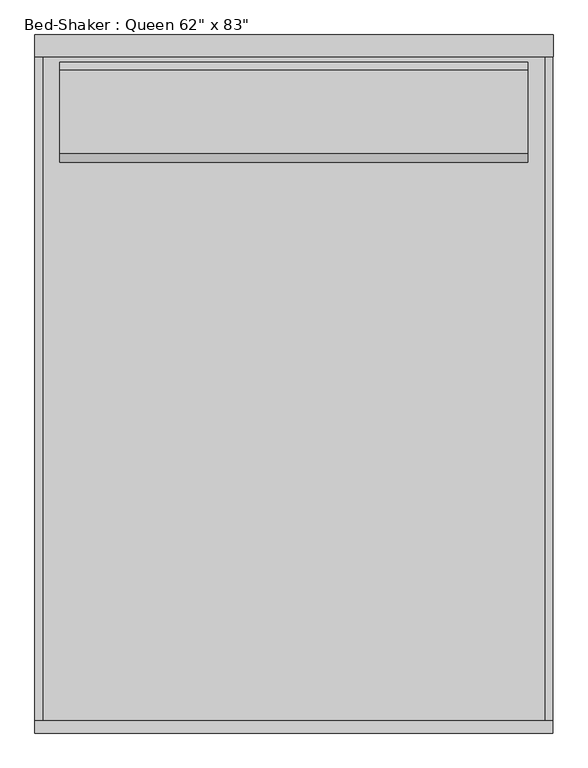
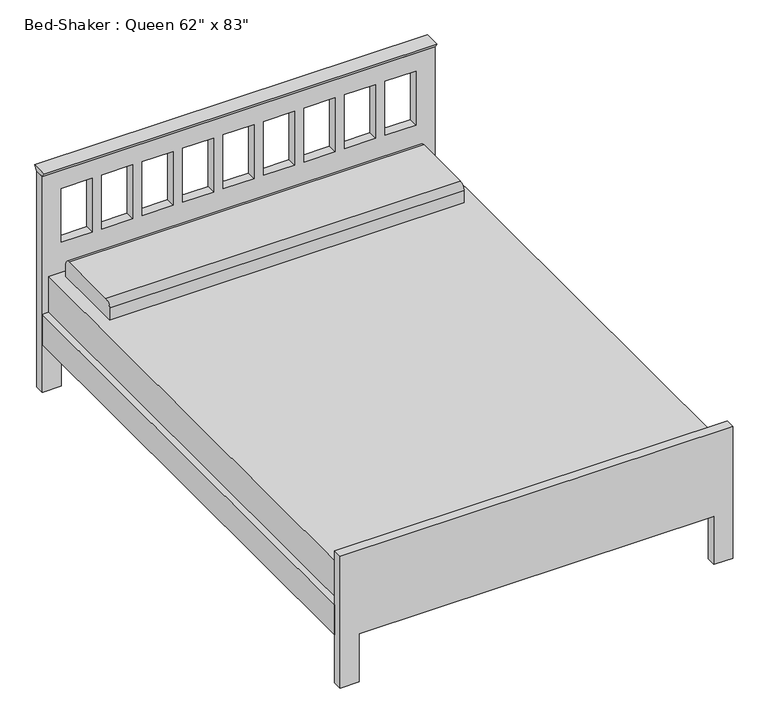
"""IFC4 building model written with IfcOpenShell, lengths in millimetres: furniture geometry."""

from ifc_helpers import new_model, si_unit, point, frame, frame_2d, origin, place, context, project, spatial, polyline, circle_curve, trimmed, segment, composite_curve, outline, extrude, source, transform, mapped, element, save


def furniture_35c09872(model_context):
    return source(origin(), model_context, "Body", "SweptSolid", [
        extrude(outline(polyline([(-38.1, 914.4), (-51.9545455, 933.45), (13.8545455, 933.45), (0.0, 914.4), (-38.1, 914.4)])), frame((-806.2365546, 0.0, 0.0), z_axis=(1.0, 0.0, 0.0), x_axis=(0.0, 1.0, 0.0)), (0.0, 0.0, 1.0), 1574.8533613),
        extrude(outline(composite_curve([segment(polyline([(-373.2486637, 482.6), (-373.2486637, 533.4)]), True, "CONTINUOUS"), segment(trimmed(circle_curve(frame_2d((-347.8486637, 533.4)), 25.4), [point((-373.2486637, 533.4))], [point((-347.8486637, 558.8))], False, "CARTESIAN"), True, "CONTINUOUS"), segment(polyline([(-347.8486637, 558.8), (-93.8486637, 558.8)]), True, "CONTINUOUS"), segment(trimmed(circle_curve(frame_2d((-93.8486637, 533.4)), 25.4), [point((-93.8486637, 558.8))], [point((-68.4486637, 533.4))], False, "CARTESIAN"), True, "CONTINUOUS"), segment(polyline([(-68.4486637, 533.4), (-68.4486637, 482.6), (-373.2486637, 482.6)]), True, "CONTINUOUS")], self_intersect=False)), frame((-730.25, 0.0, 0.0), z_axis=(1.0, 0.0, 0.0), x_axis=(0.0, 1.0, 0.0)), (0.0, 0.0, 1.0), 1422.4),
        extrude(outline(polyline([(742.95, -38.1), (742.95, -2070.1), (-781.05, -2070.1), (-781.05, -38.1), (742.95, -38.1)])), frame((0.0, 0.0, 228.6), z_axis=(0.0, 0.0, 1.0), x_axis=(1.0, 0.0, 0.0)), (0.0, 0.0, 1.0), 254.0),
        extrude(outline(polyline([(742.95, -2070.1), (742.95, -38.1), (768.35, -38.1), (768.35, -2070.1), (742.95, -2070.1)])), frame((0.0, 0.0, 203.0994861), z_axis=(0.0, 0.0, 1.0), x_axis=(1.0, 0.0, 0.0)), (0.0, 0.0, 1.0), 127.0),
        extrude(outline(polyline([(-806.45, -2070.1), (-806.45, -38.1), (-781.05, -38.1), (-781.05, -2070.1), (-806.45, -2070.1)])), frame((0.0, 0.0, 203.5755296), z_axis=(0.0, 0.0, 1.0), x_axis=(1.0, 0.0, 0.0)), (0.0, 0.0, 1.0), 127.0),
        extrude(outline(polyline([(0.0, -730.25), (203.2, -730.25), (203.2, 692.15), (0.0, 692.15), (0.0, 768.35), (558.8, 768.35), (558.8, -806.45), (0.0, -806.45), (0.0, -730.25)])), frame((0.0, -2108.2, 0.0), z_axis=(0.0, 1.0, 0.0), x_axis=(0.0, 0.0, 1.0)), (0.0, 0.0, 1.0), 38.1),
        extrude(outline(polyline([(914.4, 768.6168067), (914.4, -806.2365546), (0.0, -806.2365546), (0.0, -730.25), (203.2, -730.25), (203.2, 692.15), (0.0, 692.15), (0.0, 768.6168067), (914.4, 768.6168067)]), holes=[polyline([(838.2, -606.0722222), (609.6, -606.0722222), (609.6, -730.25), (838.2, -730.25), (838.2, -606.0722222)]), polyline([(838.2, -443.7944444), (609.6, -443.7944444), (609.6, -567.9722222), (838.2, -567.9722222), (838.2, -443.7944444)]), polyline([(838.2, -281.5166667), (609.6, -281.5166667), (609.6, -405.6944444), (838.2, -405.6944444), (838.2, -281.5166667)]), polyline([(838.2, -119.2388889), (609.6, -119.2388889), (609.6, -243.4166667), (838.2, -243.4166667), (838.2, -119.2388889)]), polyline([(838.2, 205.3166667), (609.6, 205.3166667), (609.6, 81.1388889), (838.2, 81.1388889), (838.2, 205.3166667)]), polyline([(838.2, 367.5944444), (609.6, 367.5944444), (609.6, 243.4166667), (838.2, 243.4166667), (838.2, 367.5944444)]), polyline([(838.2, 529.8722222), (609.6, 529.8722222), (609.6, 405.6944444), (838.2, 405.6944444), (838.2, 529.8722222)]), polyline([(838.2, 692.15), (609.6, 692.15), (609.6, 567.9722222), (838.2, 567.9722222), (838.2, 692.15)]), polyline([(838.2, 43.0388889), (609.6, 43.0388889), (609.6, -81.1388889), (838.2, -81.1388889), (838.2, 43.0388889)])]), frame((0.0, -38.1, 0.0), z_axis=(0.0, 1.0, 0.0), x_axis=(0.0, 0.0, 1.0)), (0.0, 0.0, 1.0), 38.1),
    ])


if __name__ == "__main__":
    model = new_model("IFC4")
    model_context = context("Model", 3, world=origin())
    ifc_project = project(units=[si_unit("LENGTHUNIT", "METRE", prefix="MILLI")], contexts=[model_context])
    site = spatial("IfcSite", under=ifc_project)
    building = spatial("IfcBuilding", under=site)
    placement = place(None, origin())
    furniture_shape = furniture_35c09872(model_context)
    element("IfcFurniture", 1, ObjectType="Bed-Shaker : Queen 62\" x 83\"", at=placement, inside=building, context=model_context, shape_type="MappedRepresentation", body=[
        mapped(furniture_shape, transform((0.0, 0.0, 0.0), x_axis=(1.0, 0.0, 0.0), y_axis=(0.0, 1.0, 0.0), z_axis=(0.0, 0.0, 1.0))),
    ])
    save(model, "model.ifc")

# Revit data of these elements
# Type "Bed-Shaker : Queen 62\" x 83\""
#   Assembly Code = "E2020200"
#   Length = 6' - 11"
#   Width = 5' - 2"
#   Frame Material = Birch
#   Mattress Material = Plywood, Sheathing
#   Default Elevation = 0
# Element 1 (IfcFurniture, "Bed-Shaker : Queen 62\" x 83\"")
#   Materials on its faces: "Birch", "Plywood, Sheathing"
# Materials
#   "Birch": class "Wood", colour RGB 210 159 95, transparency 0, Description = "Betula Alleghaniensis", Cost = 0
#   "Plywood, Sheathing": class "Wood", colour RGB 212 179 113, transparency 0, Description = "Plywood, sheathing grade", Cost = 0
